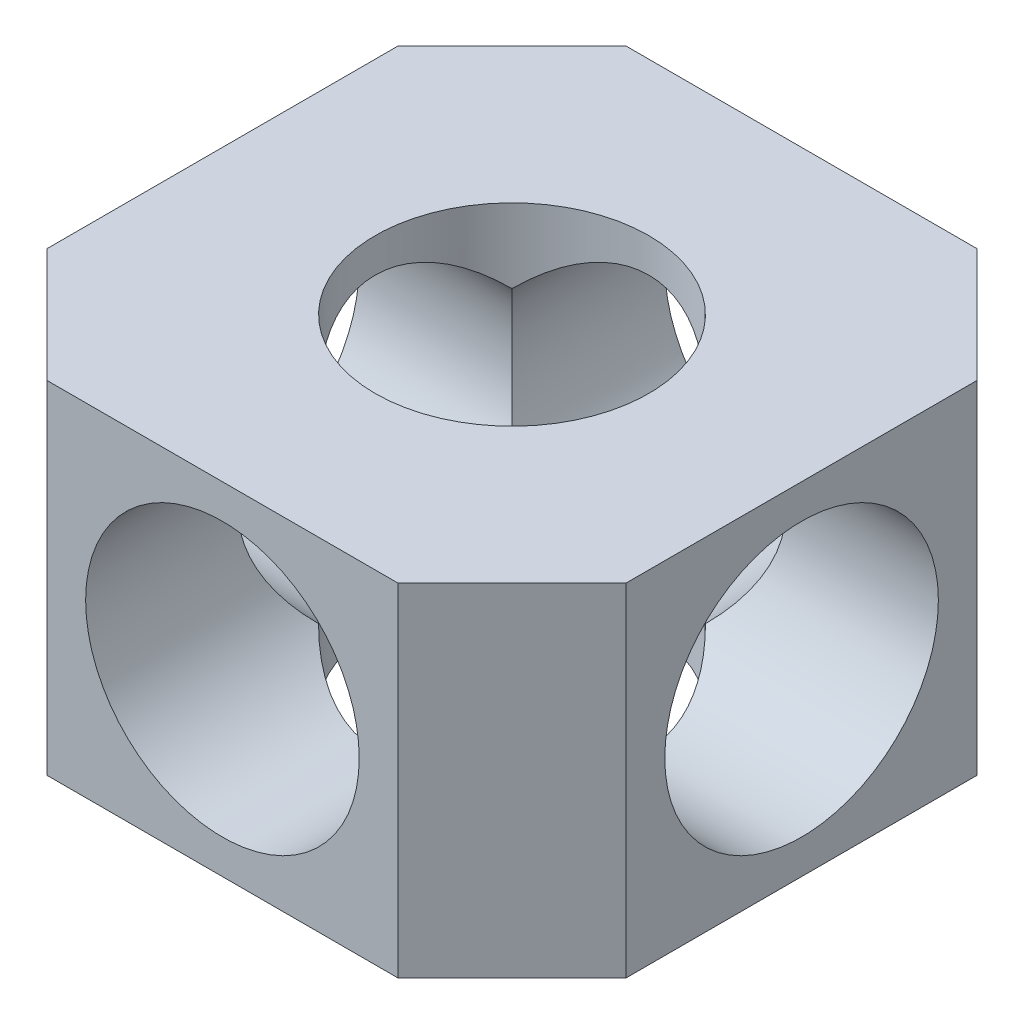
from build123d import *

# Parameters (mm, degrees)
BASE_BLOCK_DEPTH       = 15
CORNER_CHAMFER_1_SIZE  = 5
CORNER_CHAMFER_2_SIZE  = 5
CORNER_CHAMFER_3_SIZE  = 5
CORNER_CHAMFER_4_SIZE  = 5
SIDE_HOLE_A_SKETCH_R   = 6
SIDE_HOLE_A_12_DEPTH   = 36
SIDE_HOLE_B_SKETCH_R   = 6
SIDE_HOLE_B_12_DEPTH   = 36
VERTICAL_BORE_SKETCH_R = 6
VERTICAL_BORE_12_DEPTH = 36


with BuildPart() as part:
    # Base Square Sketch → Base Block (new body)
    with BuildSketch(Plane(origin=(0, 0, 0), x_dir=(1, 0, 0), z_dir=(0, 1, 0))):
        Polygon((12.7, 0), (12.7, 12.7), (-12.7, 12.7), (-12.7, -12.7), (12.7, -12.7), align=None)
    extrude(amount=BASE_BLOCK_DEPTH)

    # Corner Chamfer 1
    corner_chamfer_1_edges = [part.edges().sort_by_distance(p)[0] for p in [
        (12.7, 7.5, 12.7),
    ]]
    chamfer(corner_chamfer_1_edges, length=CORNER_CHAMFER_1_SIZE)

    # Corner Chamfer 2
    corner_chamfer_2_edges = [part.edges().sort_by_distance(p)[0] for p in [
        (12.7, 7.5, -12.7),
    ]]
    chamfer(corner_chamfer_2_edges, length=CORNER_CHAMFER_2_SIZE)

    # Corner Chamfer 3
    corner_chamfer_3_edges = [part.edges().sort_by_distance(p)[0] for p in [
        (-12.7, 7.5, -12.7),
    ]]
    chamfer(corner_chamfer_3_edges, length=CORNER_CHAMFER_3_SIZE)

    # Corner Chamfer 4
    corner_chamfer_4_edges = [part.edges().sort_by_distance(p)[0] for p in [
        (-12.7, 7.5, 12.7),
    ]]
    chamfer(corner_chamfer_4_edges, length=CORNER_CHAMFER_4_SIZE)

    # Side Hole A Sketch → Side Hole A Ø12 (cut)
    with BuildSketch(Plane(origin=(0, 0, -12.7), x_dir=(-1, 0, 0), z_dir=(0, 0, -1))):
        with Locations((0, 7.5)):
            Circle(SIDE_HOLE_A_SKETCH_R)
    extrude(amount=-SIDE_HOLE_A_12_DEPTH, mode=Mode.SUBTRACT)

    # Side Hole B Sketch → Side Hole B Ø12 (cut)
    with BuildSketch(Plane(origin=(12.7, 0, 0), x_dir=(0, 0, -1), z_dir=(1, 0, 0))):
        with Locations((0, 7.5)):
            Circle(SIDE_HOLE_B_SKETCH_R)
    extrude(amount=-SIDE_HOLE_B_12_DEPTH, mode=Mode.SUBTRACT)

    # Vertical Bore Sketch → Vertical Bore Ø12 (cut)
    with BuildSketch(Plane(origin=(0, 15, 0), x_dir=(1, 0, 0), z_dir=(0, 1, 0))):
        with Locations(Location((0, 0, 0), (0, 0, 270))):
            Circle(VERTICAL_BORE_SKETCH_R)
    extrude(amount=-VERTICAL_BORE_12_DEPTH, mode=Mode.SUBTRACT)


solid = part.part
